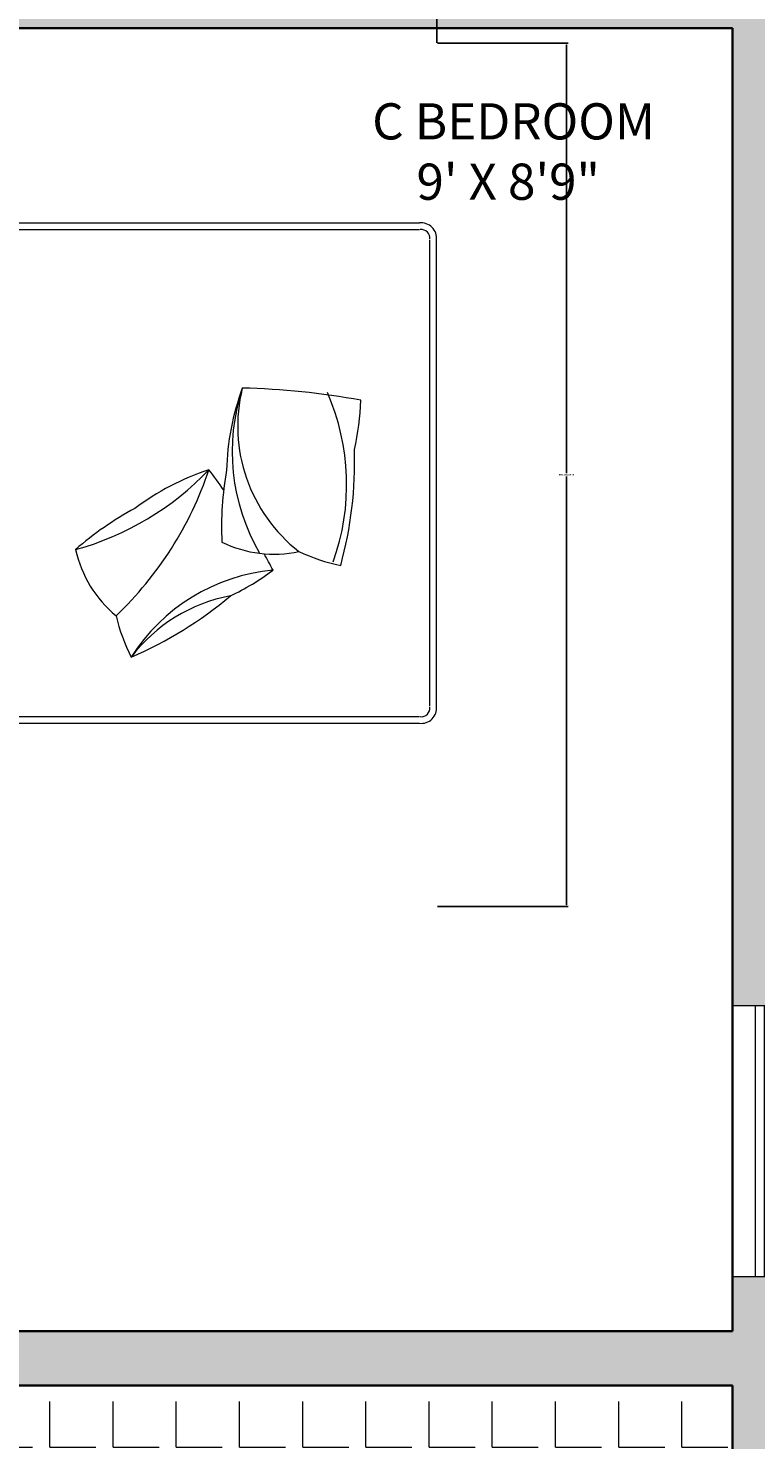
# Model space of a CAD drawing. Units: inches. Extents: x 2701 to 6846, y 811 to 2447.
# Tile 18 of 20: x 3008 to 3089, y 1300 to 1456. Entities that reach past the tile are written whole.
import ezdxf

# ---------------------------------------------------------------- set-up
doc = ezdxf.new("R2010")
doc.units = ezdxf.units.IN
for name, color, linetype, lineweight in [('A-ANNO-DIMS', 2, 'Continuous', 18), ('A-AREA-IDEN', 7, 'Continuous', 18), ('A-FLOR-PATT', 252, 'Continuous', 13), ('A-FURN', 8, 'Continuous', 13), ('A-GLAZ', 4, 'Continuous', 18), ('A-WALL', 7, 'Continuous', 35)]:
    doc.layers.add(name, color=color, linetype=linetype, lineweight=lineweight)
doc.layers.add('A-WALL-PATT', color=18, linetype='Continuous', lineweight=13, true_color=0x000000)
doc.styles.get("Standard").update_dxf_attribs({"font": 'arial.ttf'})
doc.dimstyles.get("Standard").update_dxf_attribs({"dimtxt": 0.18, "dimasz": 0.18, "dimexe": 0.18, "dimexo": 0.0625, "dimgap": 0.09, "dimtad": 0, "dimtih": 1, "dimtoh": 1, "dimdec": 4, "dimzin": 0, "dimdsep": 46, "dimtxsty": 'Standard', "dimcen": 0.09, "dimadec": 0, "dimazin": 0, "dimtfac": 1, "dimtdec": 4, "dimtofl": 0, "dimtmove": 0, "dimatfit": 3, "dimfxl": 1, "dimtolj": 1, "dimtzin": 0, "dimarcsym": 0})

# ---------------------------------------------------------------- blocks, each defined once
blk = doc.blocks.new('W1')
for p, q in [((3091.97, 1348.05), (3091.97, 1360.05)), ((3091.97, 1360.05), (3091.97, 1358.83)), ((3091.97, 1360.05), (3101.22, 1360.05)), ((3101.22, 1306.05), (3101.22, 1360.05)), ((3085.97, 1318.05), (3085.97, 1348.05)), ((3085.97, 1348.05), (3091.97, 1348.05)), ((3088.47, 1348.05), (3088.47, 1318.05)), ((3089.47, 1348.05), (3089.47, 1318.05)), ((3091.97, 1348.05), (3091.97, 1348.05)), ((3091.97, 1348.05), (3091.97, 1318.05)), ((3091.97, 1318.05), (3085.97, 1318.05)), ((3091.97, 1318.05), (3091.97, 1306.05)), ((3091.97, 1306.05), (3091.97, 1306.05)), ((3091.97, 1306.05), (3101.22, 1306.05))]:
    blk.add_line(p, q)
blk.add_circle((3096.65, 1332.84), 3.33)
at = {"insert": (3097.78, 1330.51), "char_height": 2.5, "attachment_point": 7, "rotation": 90}
blk.add_mtext('W1', dxfattribs=at)
blk = doc.blocks.new('A$C356F0359')
for p, q in [((0.5489, 2), (2.0492, 2)), ((0.5489, 1.9489), (0.5489, 2)), ((2.0492, 1.9489), (2.0492, 2)), ((0.4398, 1.9801), (0.0598, 1.9801)), ((0.4398, 1.9601), (0.0598, 1.9601)), ((2.0492, 1.9489), (0.5489, 1.9489)), ((2.5283, 1.9801), (2.1483, 1.9801)), ((2.5283, 1.9601), (2.1483, 1.9601)), ((-0.0002, 1.9201), (-0.0002, 1.5401)), ((0.0198, 1.9201), (0.0198, 1.5401)), ((0.4798, 1.5401), (0.4798, 1.9201)), ((0.4998, 1.5401), (0.4998, 1.9201)), ((1.998, 1.9289), (0.6001, 1.9289)), ((2.0883, 1.9201), (2.0883, 1.5401)), ((2.1083, 1.9201), (2.1083, 1.5401)), ((2.5683, 1.5401), (2.5683, 1.9201)), ((2.5883, 1.5401), (2.5883, 1.9201)), ((0.1539, 1.5681), (0.1539, 1.8777)), ((0.2725, 1.8879), (0.2702, 1.8856)), ((0.2702, 1.8856), (0.2702, 1.7279)), ((0.2725, 1.8879), (0.4531, 1.8879)), ((0.3913, 1.8753), (0.277, 1.8753)), ((0.277, 1.8753), (0.277, 1.8147)), ((0.3913, 1.8147), (0.3913, 1.8753)), ((0.4016, 1.8787), (0.4062, 1.8845)), ((0.4016, 1.7404), (0.4016, 1.8787)), ((0.4062, 1.881), (0.405, 1.8765)), ((0.405, 1.8765), (0.4153, 1.8662)), ((0.405, 1.8765), (0.405, 1.8456)), ((0.4062, 1.8845), (0.4405, 1.8845)), ((0.4108, 1.8833), (0.4062, 1.881)), ((0.4108, 1.8833), (0.4382, 1.8833)), ((0.4165, 1.8685), (0.4108, 1.8833)), ((0.4153, 1.8662), (0.4165, 1.8685)), ((0.4153, 1.8147), (0.4153, 1.8662)), ((0.4325, 1.8685), (0.4165, 1.8685)), ((0.4325, 1.8685), (0.4382, 1.8833)), ((0.4336, 1.8662), (0.4325, 1.8685)), ((0.4439, 1.8765), (0.4336, 1.8662)), ((0.4336, 1.8147), (0.4336, 1.8662)), ((0.4382, 1.8833), (0.4428, 1.881)), ((0.4405, 1.8845), (0.4462, 1.8787)), ((0.4428, 1.881), (0.4439, 1.8765)), ((0.4439, 1.8765), (0.4439, 1.8456)), ((0.4462, 1.8787), (0.4462, 1.7416)), ((0.4531, 1.8879), (0.4553, 1.8856)), ((0.4553, 1.8856), (0.4553, 1.7279)), ((0.5489, 1.8977), (0.5489, 0.0512)), ((0.5689, 1.8977), (0.5689, 0.0512)), ((2.0292, 0.0512), (2.0292, 1.8977)), ((2.0492, 0.0512), (2.0492, 1.8977)), ((2.3306, 1.5822), (2.3306, 1.8917)), ((0.405, 1.8456), (0.4073, 1.8399)), ((0.4073, 1.8399), (0.4108, 1.8342)), ((0.4108, 1.8342), (0.4119, 1.8262)), ((0.4119, 1.8262), (0.4119, 1.8147)), ((0.4382, 1.8342), (0.4371, 1.8262)), ((0.4371, 1.8262), (0.4371, 1.8147)), ((0.4416, 1.8399), (0.4382, 1.8342)), ((0.4439, 1.8456), (0.4416, 1.8399)), ((0.277, 1.8147), (0.3913, 1.8147)), ((0.277, 1.7885), (0.277, 1.7679)), ((0.3445, 1.7885), (0.277, 1.7885)), ((0.3913, 1.8125), (0.2816, 1.8125)), ((0.2816, 1.8125), (0.2816, 1.801)), ((0.2816, 1.801), (0.3913, 1.801)), ((0.2885, 1.7862), (0.2885, 1.7827)), ((0.2919, 1.7862), (0.2885, 1.7862)), ((0.2885, 1.7827), (0.2919, 1.7827)), ((0.2907, 1.8125), (0.2907, 1.801)), ((0.2919, 1.7827), (0.2919, 1.7862)), ((0.2999, 1.8125), (0.2999, 1.801)), ((0.309, 1.8125), (0.309, 1.801)), ((0.3125, 1.7862), (0.309, 1.7862)), ((0.309, 1.7862), (0.309, 1.7827)), ((0.309, 1.7827), (0.3125, 1.7827)), ((0.3125, 1.7827), (0.3125, 1.7862)), ((0.3182, 1.8125), (0.3182, 1.801)), ((0.3273, 1.8125), (0.3273, 1.801)), ((0.333, 1.7862), (0.3296, 1.7862)), ((0.3296, 1.7862), (0.3296, 1.7827)), ((0.3296, 1.7827), (0.333, 1.7827)), ((0.333, 1.7827), (0.333, 1.7862)), ((0.3365, 1.8125), (0.3365, 1.801)), ((0.3445, 1.7679), (0.3445, 1.7885)), ((0.3548, 1.7759), (0.3548, 1.7827)), ((0.3548, 1.7827), (0.3639, 1.7827)), ((0.3639, 1.7827), (0.3639, 1.7759)), ((0.3685, 1.7827), (0.3776, 1.7827)), ((0.3685, 1.7759), (0.3685, 1.7827)), ((0.3776, 1.7827), (0.3776, 1.7759)), ((0.3822, 1.7759), (0.3822, 1.7827)), ((0.3822, 1.7827), (0.3913, 1.7827)), ((0.3913, 1.801), (0.3913, 1.8125)), ((0.3913, 1.7827), (0.3913, 1.7759)), ((0.405, 1.7736), (0.4073, 1.7793)), ((0.4073, 1.7793), (0.4108, 1.785)), ((0.4108, 1.785), (0.4119, 1.793)), ((0.4119, 1.793), (0.4119, 1.8147)), ((0.4153, 1.8147), (0.4153, 1.753)), ((0.4336, 1.8147), (0.4336, 1.753)), ((0.4371, 1.793), (0.4371, 1.8147)), ((0.4382, 1.785), (0.4371, 1.793)), ((0.4416, 1.7793), (0.4382, 1.785)), ((0.4439, 1.7736), (0.4416, 1.7793)), ((0.277, 1.7679), (0.3445, 1.7679)), ((0.2782, 1.7622), (0.2782, 1.7576)), ((0.2896, 1.7622), (0.2782, 1.7622)), ((0.2782, 1.7576), (0.2896, 1.7576)), ((0.2782, 1.745), (0.2896, 1.745)), ((0.2782, 1.7382), (0.2782, 1.745)), ((0.2896, 1.7382), (0.2782, 1.7382)), ((0.2919, 1.7736), (0.2885, 1.7736)), ((0.2885, 1.7736), (0.2885, 1.7702)), ((0.2885, 1.7702), (0.2919, 1.7702)), ((0.2896, 1.7576), (0.2896, 1.7622)), ((0.2896, 1.745), (0.2896, 1.7382)), ((0.2919, 1.7702), (0.2919, 1.7736)), ((0.2942, 1.7622), (0.2942, 1.7576)), ((0.3056, 1.7622), (0.2942, 1.7622)), ((0.2942, 1.7576), (0.3056, 1.7576)), ((0.2942, 1.745), (0.3056, 1.745)), ((0.2942, 1.7382), (0.2942, 1.745)), ((0.3056, 1.7382), (0.2942, 1.7382)), ((0.3056, 1.7576), (0.3056, 1.7622)), ((0.3056, 1.745), (0.3056, 1.7382)), ((0.3125, 1.7736), (0.309, 1.7736)), ((0.309, 1.7736), (0.309, 1.7702)), ((0.309, 1.7702), (0.3125, 1.7702)), ((0.3102, 1.7622), (0.3102, 1.7576)), ((0.3216, 1.7622), (0.3102, 1.7622)), ((0.3102, 1.7576), (0.3216, 1.7576)), ((0.3102, 1.745), (0.3216, 1.745)), ((0.3102, 1.7382), (0.3102, 1.745)), ((0.3216, 1.7382), (0.3102, 1.7382)), ((0.3125, 1.7702), (0.3125, 1.7736)), ((0.3216, 1.7576), (0.3216, 1.7622)), ((0.3216, 1.745), (0.3216, 1.7382)), ((0.3376, 1.7622), (0.3262, 1.7622)), ((0.3262, 1.7622), (0.3262, 1.7576)), ((0.3262, 1.7576), (0.3376, 1.7576)), ((0.3262, 1.7382), (0.3262, 1.745)), ((0.3262, 1.745), (0.3376, 1.745)), ((0.3376, 1.7382), (0.3262, 1.7382)), ((0.333, 1.7736), (0.3296, 1.7736)), ((0.3296, 1.7736), (0.3296, 1.7702)), ((0.3296, 1.7702), (0.333, 1.7702)), ((0.333, 1.7702), (0.333, 1.7736)), ((0.3376, 1.7576), (0.3376, 1.7622)), ((0.3376, 1.745), (0.3376, 1.7382)), ((0.3639, 1.7759), (0.3548, 1.7759)), ((0.3548, 1.7633), (0.3548, 1.7702)), ((0.3548, 1.7702), (0.3639, 1.7702)), ((0.3639, 1.7633), (0.3548, 1.7633)), ((0.3548, 1.7564), (0.3639, 1.7564)), ((0.3548, 1.7496), (0.3548, 1.7564)), ((0.3639, 1.7496), (0.3548, 1.7496)), ((0.3548, 1.737), (0.3548, 1.7439)), ((0.3548, 1.7439), (0.3639, 1.7439)), ((0.3639, 1.737), (0.3548, 1.737)), ((0.3639, 1.7702), (0.3639, 1.7633)), ((0.3639, 1.7564), (0.3639, 1.7496)), ((0.3639, 1.7439), (0.3639, 1.737)), ((0.3776, 1.7759), (0.3685, 1.7759)), ((0.3685, 1.7633), (0.3685, 1.7702)), ((0.3685, 1.7702), (0.3776, 1.7702)), ((0.3776, 1.7633), (0.3685, 1.7633)), ((0.3685, 1.7564), (0.3776, 1.7564)), ((0.3685, 1.7496), (0.3685, 1.7564)), ((0.3776, 1.7496), (0.3685, 1.7496)), ((0.3685, 1.737), (0.3685, 1.7439)), ((0.3685, 1.7439), (0.3776, 1.7439)), ((0.3776, 1.737), (0.3685, 1.737)), ((0.3776, 1.7702), (0.3776, 1.7633)), ((0.3776, 1.7564), (0.3776, 1.7496)), ((0.3776, 1.7439), (0.3776, 1.737)), ((0.3913, 1.7759), (0.3822, 1.7759)), ((0.3822, 1.7633), (0.3822, 1.7702)), ((0.3822, 1.7702), (0.3913, 1.7702)), ((0.3913, 1.7633), (0.3822, 1.7633)), ((0.3822, 1.7576), (0.3913, 1.7576)), ((0.3822, 1.7507), (0.3822, 1.7576)), ((0.3913, 1.7507), (0.3822, 1.7507)), ((0.3822, 1.7439), (0.3913, 1.7439)), ((0.3822, 1.737), (0.3822, 1.7439)), ((0.3913, 1.737), (0.3822, 1.737)), ((0.3913, 1.7702), (0.3913, 1.7633)), ((0.3913, 1.7576), (0.3913, 1.7507)), ((0.3913, 1.7439), (0.3913, 1.737)), ((0.4073, 1.7347), (0.4016, 1.7404)), ((0.405, 1.7427), (0.405, 1.7736)), ((0.405, 1.7427), (0.4153, 1.753)), ((0.4062, 1.7382), (0.405, 1.7427)), ((0.4108, 1.7359), (0.4062, 1.7382)), ((0.4165, 1.7507), (0.4108, 1.7359)), ((0.4108, 1.7359), (0.4234, 1.7359)), ((0.4153, 1.753), (0.4165, 1.7507)), ((0.4325, 1.7507), (0.4165, 1.7507)), ((0.4233, 1.7393), (0.4235, 1.7294)), ((0.4268, 1.7393), (0.4233, 1.7393)), ((0.4274, 1.7301), (0.4268, 1.7393)), ((0.427, 1.7359), (0.4382, 1.7359)), ((0.4336, 1.753), (0.4325, 1.7507)), ((0.4325, 1.7507), (0.4382, 1.7359)), ((0.4439, 1.7427), (0.4336, 1.753)), ((0.4382, 1.7359), (0.4428, 1.7382)), ((0.4462, 1.7416), (0.4405, 1.7347)), ((0.4428, 1.7382), (0.4439, 1.7427)), ((0.4439, 1.7427), (0.4439, 1.7736)), ((0.4622, 1.7459), (0.4553, 1.7484)), ((0.4553, 1.7439), (0.4604, 1.7425)), ((0.4604, 1.7425), (0.465, 1.7388)), ((0.4654, 1.7427), (0.4622, 1.7459)), ((0.465, 1.7388), (0.4662, 1.7372)), ((0.4678, 1.7405), (0.4654, 1.7427)), ((0.4662, 1.7372), (0.4686, 1.7374)), ((0.4686, 1.7374), (0.4662, 1.735)), ((0.4721, 1.7421), (0.4678, 1.7405)), ((0.4741, 1.7401), (0.4721, 1.7421)), ((0.4725, 1.7366), (0.4741, 1.7401)), ((0.4753, 1.7388), (0.4725, 1.7366)), ((0.4783, 1.7356), (0.4753, 1.7388)), ((2.4819, 1.7366), (2.1818, 1.7366)), ((0.3052, 1.7226), (0.0051, 1.7226)), ((0.2702, 1.7279), (0.2725, 1.7256)), ((0.4244, 1.7256), (0.2725, 1.7256)), ((0.4234, 1.7347), (0.4073, 1.7347)), ((0.4235, 1.7294), (0.4263, 1.7179)), ((0.4263, 1.7179), (0.429, 1.707)), ((0.427, 1.697), (0.4265, 1.6915)), ((0.4295, 1.6996), (0.427, 1.697)), ((0.4405, 1.7347), (0.4271, 1.7347)), ((0.429, 1.7227), (0.4274, 1.7301)), ((0.4531, 1.7256), (0.4284, 1.7256)), ((0.429, 1.707), (0.4288, 1.701)), ((0.4288, 1.701), (0.4295, 1.6996)), ((0.4318, 1.7119), (0.429, 1.7227)), ((0.4325, 1.7063), (0.4318, 1.7119)), ((0.4323, 1.7003), (0.4325, 1.7063)), ((0.4364, 1.6973), (0.4323, 1.7003)), ((0.4355, 1.6919), (0.4364, 1.6973)), ((0.4553, 1.7279), (0.4531, 1.7256)), ((0.4662, 1.735), (0.4755, 1.7268)), ((0.4755, 1.7268), (0.4906, 1.7139)), ((0.4759, 1.729), (0.4783, 1.7356)), ((0.4821, 1.7322), (0.4759, 1.729)), ((0.4874, 1.7272), (0.4821, 1.7322)), ((0.4862, 1.7199), (0.4874, 1.7272)), ((0.4914, 1.7231), (0.4862, 1.7199)), ((0.4908, 1.7135), (0.4984, 1.6917)), ((0.4958, 1.7185), (0.4914, 1.7231)), ((0.494, 1.7135), (0.4958, 1.7185)), ((0.501, 1.7142), (0.494, 1.7135)), ((0.4964, 1.7047), (0.5031, 1.7072)), ((0.5038, 1.7049), (0.4964, 1.7047)), ((0.5005, 1.695), (0.5054, 1.6996)), ((0.5068, 1.695), (0.5005, 1.695)), ((0.5031, 1.7072), (0.501, 1.7142)), ((0.5054, 1.6996), (0.5038, 1.7049)), ((0.5079, 1.6892), (0.5068, 1.695)), ((0.4265, 1.6915), (0.4332, 1.6903)), ((0.4332, 1.6903), (0.4267, 1.6864)), ((0.4267, 1.6864), (0.4272, 1.6801)), ((0.4272, 1.6801), (0.4346, 1.6794)), ((0.4346, 1.6794), (0.4281, 1.6744)), ((0.4281, 1.6744), (0.4311, 1.669)), ((0.4311, 1.669), (0.4381, 1.6704)), ((0.4381, 1.6704), (0.4348, 1.6639)), ((0.4348, 1.6639), (0.4383, 1.6598)), ((0.4367, 1.6774), (0.4355, 1.6919)), ((0.4455, 1.6663), (0.4367, 1.6774)), ((0.4383, 1.6598), (0.4436, 1.6637)), ((0.4436, 1.6637), (0.4427, 1.6575)), ((0.4427, 1.6575), (0.4471, 1.6547)), ((0.4577, 1.6598), (0.4455, 1.6663)), ((0.4471, 1.6547), (0.4526, 1.6593)), ((0.4526, 1.6593), (0.4519, 1.6517)), ((0.4519, 1.6517), (0.4568, 1.6503)), ((0.4568, 1.6503), (0.4598, 1.6565)), ((0.4716, 1.6586), (0.4577, 1.6598)), ((0.4598, 1.6565), (0.4626, 1.6503)), ((0.4665, 1.6498), (0.4681, 1.6565)), ((0.4681, 1.6565), (0.4707, 1.6491)), ((0.485, 1.6644), (0.4716, 1.6586)), ((0.4751, 1.6503), (0.4753, 1.6565)), ((0.4753, 1.6565), (0.4806, 1.6519)), ((0.4806, 1.6519), (0.4843, 1.6538)), ((0.4843, 1.6538), (0.4836, 1.6607)), ((0.4836, 1.6607), (0.4885, 1.6547)), ((0.4952, 1.6744), (0.485, 1.6644)), ((0.4885, 1.6547), (0.4922, 1.6579)), ((0.4922, 1.6579), (0.4894, 1.6642)), ((0.4894, 1.6642), (0.4959, 1.6614)), ((0.4984, 1.6917), (0.4952, 1.6744)), ((0.4957, 1.6704), (0.5024, 1.6683)), ((0.4989, 1.6642), (0.4957, 1.6704)), ((0.4959, 1.6614), (0.4989, 1.6642)), ((0.5042, 1.673), (0.4987, 1.6792)), ((0.4987, 1.6792), (0.5058, 1.679)), ((0.5008, 1.6871), (0.5079, 1.6892)), ((0.5068, 1.6836), (0.5008, 1.6871)), ((0.5024, 1.6683), (0.5042, 1.673)), ((0.5058, 1.679), (0.5068, 1.6836)), ((0.4626, 1.6503), (0.4665, 1.6498)), ((0.4707, 1.6491), (0.4751, 1.6503)), ((0.0598, 1.5001), (0.4398, 1.5001)), ((2.1483, 1.5001), (2.5283, 1.5001)), ((0.0598, 1.4801), (0.4398, 1.4801)), ((2.1483, 1.4801), (2.5283, 1.4801)), ((0.6001, 0.02), (1.998, 0.02)), ((0.6001, 0), (1.998, 0))]:
    blk.add_line(p, q)
at = {"linetype": 'ByBlock'}
for p, q in [((0.6001, 1.9147), (1.282, 1.9147)), ((0.6001, 1.6759), (0.6001, 1.9147)), ((1.282, 1.9147), (1.282, 1.6759)), ((1.3161, 1.9147), (1.998, 1.9147)), ((1.3161, 1.6759), (1.3161, 1.9147)), ((1.998, 1.9147), (1.998, 1.6759)), ((1.282, 1.6759), (0.6001, 1.6759)), ((1.998, 1.6759), (1.3161, 1.6759)), ((1.0687, 1.6418), (0.5489, 1.6418)), ((1.4185, 1.5053), (0.5489, 1.5053))]:
    blk.add_line(p, q, dxfattribs=at)
for centre in [(0.1539, 1.7226), (2.3306, 1.7366)]:
    blk.add_circle(centre, 0.12, dxfattribs=at)
for centre in [(0.1539, 1.7226), (2.3306, 1.7366)]:
    blk.add_circle(centre, 0.06)
for centre, radius, start, end in [((0.0598, 1.9201), 0.06, 90, 180), ((0.0598, 1.9201), 0.04, 90, 180), ((0.4398, 1.9201), 0.06, 0, 90), ((0.4398, 1.9201), 0.04, 0, 90), ((0.6001, 1.8977), 0.0512, 90, 180), ((1.998, 1.8977), 0.0512, 0, 90), ((2.1483, 1.9201), 0.06, 90, 180), ((2.1483, 1.9201), 0.04, 90, 180), ((2.5283, 1.9201), 0.06, 0, 90), ((2.5283, 1.9201), 0.04, 0, 90), ((0.6001, 1.8977), 0.0312, 90, 180), ((1.998, 1.8977), 0.0312, 0, 90), ((0.0598, 1.5401), 0.06, 180, 270), ((0.0598, 1.5401), 0.04, 180, 270), ((0.4398, 1.5401), 0.04, 270, 0), ((0.4398, 1.5401), 0.06, 270, 0), ((2.1483, 1.5401), 0.06, 180, 270), ((2.1483, 1.5401), 0.04, 180, 270), ((2.5283, 1.5401), 0.06, 270, 0), ((2.5283, 1.5401), 0.04, 270, 0), ((1.1471, 0.7332), 0.3575, 102.4782, 140.4625), ((1.9086, 1.3124), 0.8697, 195.336, 226.4193), ((0.3249, 0.4335), 0.9879, 28.4971, 41.0566), ((0.9965, 0.4273), 0.548, 103.2034, 117.0362), ((1.6529, 1.7059), 1.0798, 223.6306, 251.4288), ((0.4451, 0.4375), 0.5655, 5.3391, 57.6895), ((0.4517, 0.5274), 0.4879, 10.6986, 52.6864), ((1.8195, 1.3719), 1.1652, 203.0642, 220.3209), ((0.5617, 0.4344), 0.7874, 18.3527, 36.6851), ((-0.021, 2.4319), 2.1977, 305.2966, 307.2418), ((1.4135, 0.487), 0.3575, 154.0418, 192.0262), ((1.1372, -0.3434), 0.9879, 80.0607, 92.6202), ((1.5949, 0.9312), 0.734, 205.259, 216.9351), ((1.3641, 0.0041), 0.6085, 71.81, 120.1351), ((1.44, 0.1186), 0.4774, 76.1849, 142.0017), ((1.2836, -0.1573), 0.7874, 69.9163, 88.2487), ((-0.6432, 0.628), 2.1977, 349.4884, 358.8054), ((-0.021, 2.4319), 2.1977, 297.9248, 299.3793), ((1.5595, 0.1789), 0.548, 154.767, 168.5998), ((1.2647, 0.9578), 0.6885, 250.2936, 293.6414), ((1.3312, 1.4107), 1.1652, 254.6278, 271.8845), ((1.5368, 0.9609), 0.734, 256.8226, 268.4988), ((0.5943, 0.0454), 0.0458, 172.7599, 277.2401), ((0.5943, 0.0454), 0.0258, 172.7599, 277.2401), ((2.0038, 0.0454), 0.0458, 262.7599, 7.2401), ((2.0038, 0.0454), 0.0258, 262.7599, 7.2401)]:
    blk.add_arc(centre, radius, start, end)
for centre, radius, start, end in [((0.1906, 1.7953), 0.4265, 343.7398, 16.2602), ((1.6914, 1.7953), 0.4265, 163.7398, 196.2602), ((0.9067, 1.7953), 0.4265, 343.7398, 16.2602), ((2.4075, 1.7953), 0.4265, 163.7398, 196.2602), ((0.9303, 0.657), 0.9853, 61.4328, 88.1261), ((1.0826, 0.5712), 1.0706, 72.1966, 90.7418), ((2.1368, 4.5996), 3.0955, 256.4201, 268.3789), ((2.0056, 2.7745), 1.3903, 244.2427, 271.7984)]:
    blk.add_arc(centre, radius, start, end, dxfattribs=at)
blk = doc.blocks.new('*D34')
at = {"layer": 'A-ANNO-DIMS', "color": 0, "lineweight": -2, "transparency": 16777216}
for p, q in [((3085.97, 1305.99), (3085.97, 1297.77)), ((3101.22, 1305.99), (3101.22, 1297.77)), ((3086.15, 1297.95), (3093.38, 1297.95)), ((3101.04, 1297.95), (3093.81, 1297.95))]:
    blk.add_line(p, q, dxfattribs=at)
at = {"layer": 'A-ANNO-DIMS', "color": 0, "transparency": 16777216}
for points in [[(3086.15, 1297.98), (3086.15, 1297.92), (3085.97, 1297.95)], [(3101.04, 1297.98), (3101.04, 1297.92), (3101.22, 1297.95)]]:
    blk.add_solid(points, dxfattribs=at)
at = {"layer": 'Defpoints', "color": 0, "transparency": 16777216}
for p in [(3085.97, 1306.05), (3101.22, 1306.05), (3101.22, 1297.95)]:
    blk.add_point(p, dxfattribs=at)
at = {"layer": 'A-ANNO-DIMS', "color": 0, "transparency": 16777216, "insert": (3093.59, 1297.95), "char_height": 0.18, "attachment_point": 5}
blk.add_mtext('\\A1;15', dxfattribs=at)
blk = doc.blocks.new('*D51')
at = {"layer": 'A-ANNO-DIMS', "color": 0, "lineweight": -2, "transparency": 16777216}
for p, q in [((3053.38, 1454.39), (3067.81, 1454.39)), ((3067.63, 1454.21), (3067.63, 1406.88)), ((3067.63, 1359.18), (3067.63, 1406.51)), ((3053.38, 1359), (3067.81, 1359))]:
    blk.add_line(p, q, dxfattribs=at)
at = {"layer": 'A-ANNO-DIMS', "color": 0, "transparency": 16777216}
for points in [[(3067.6, 1454.21), (3067.66, 1454.21), (3067.63, 1454.39)], [(3067.6, 1359.18), (3067.66, 1359.18), (3067.63, 1359)]]:
    blk.add_solid(points, dxfattribs=at)
at = {"layer": 'Defpoints', "color": 0, "transparency": 16777216}
for p in [(3053.32, 1454.39), (3067.63, 1454.39), (3053.32, 1359)]:
    blk.add_point(p, dxfattribs=at)
at = {"layer": 'A-ANNO-DIMS', "color": 0, "transparency": 16777216, "insert": (3067.63, 1406.69), "char_height": 0.18, "attachment_point": 5}
blk.add_mtext('\\A1;BED GROUP 95', dxfattribs=at)
blk = doc.blocks.new('*D52')
at = {"layer": 'A-ANNO-DIMS', "color": 0, "lineweight": -2, "transparency": 16777216}
for p, q in [((2979.55, 1454.45), (2979.55, 1468.88)), ((2979.73, 1468.7), (3016.22, 1468.7)), ((3053.14, 1468.7), (3016.65, 1468.7)), ((3053.32, 1454.45), (3053.32, 1468.88))]:
    blk.add_line(p, q, dxfattribs=at)
at = {"layer": 'A-ANNO-DIMS', "color": 0, "transparency": 16777216}
for points in [[(2979.73, 1468.73), (2979.73, 1468.67), (2979.55, 1468.7)], [(3053.14, 1468.73), (3053.14, 1468.67), (3053.32, 1468.7)]]:
    blk.add_solid(points, dxfattribs=at)
at = {"layer": 'Defpoints', "color": 0, "transparency": 16777216}
for p in [(2979.55, 1468.7), (2979.55, 1454.39), (3053.32, 1454.39)]:
    blk.add_point(p, dxfattribs=at)
at = {"layer": 'A-ANNO-DIMS', "color": 0, "transparency": 16777216, "insert": (3016.44, 1468.7), "char_height": 0.18, "attachment_point": 5}
blk.add_mtext('\\A1;74', dxfattribs=at)

msp = doc.modelspace()

# ---------------------------------------------------------------- hatches: boundary and pattern name
at = {"layer": 'A-FLOR-PATT'}
h = msp.add_hatch(dxfattribs=at)
h.set_pattern_fill('ANGLE', color=256)
h.set_pattern_definition([(0, (0, 0), (0, 6.985), [5.08, -1.905]), (90, (0, 0), (-6.985, 4e-16), [5.08, -1.905])])
h.paths.add_polyline_path([(2841.81, 1296.51, -0.109453), (2842.61, 1300.13, -0.102375), (2844.98, 1303.3, -0.093743), (2848.43, 1305.37, -0.062463), (2851.37, 1306.05), (2785.97, 1306.05), (2785.97, 1258.05), (2827.97, 1258.05), (2827.97, 1256.41), (2829.45, 1256.41, -0.394827), (2854.75, 1283.45), (2856.49, 1283.45), (2856.49, 1256.41), (2857.97, 1256.41), (2857.97, 1258.05), (2863.97, 1258.05), (2863.97, 1306.05), (2853.87, 1306.05, -0.062463), (2856.81, 1305.37, -0.093743), (2860.26, 1303.3, -0.102375), (2862.62, 1300.13, -0.109453), (2863.42, 1296.51, -0.109453), (2862.62, 1292.89, -0.102375), (2860.26, 1289.72, -0.093738), (2856.81, 1287.65, -0.088425), (2852.62, 1286.91, -0.088425), (2848.43, 1287.65, -0.093738), (2844.98, 1289.72, -0.102375), (2842.61, 1292.89, -0.109453)])
h.paths.add_polyline_path([(2805.21, 1273.88, -0.141745), (2808.32, 1271.77, -0.184983), (2809.77, 1267.97, -0.184983), (2808.32, 1264.18, -0.141745), (2805.21, 1262.07, -0.152244), (2799.99, 1261.8, -0.025614), (2799.37, 1261.95), (2794.37, 1263.42), (2794.36, 1263.41, -0.111242), (2793.99, 1261.92, -0.033889), (2793.11, 1260.11, -0.286745), (2792.38, 1259.65), (2787.58, 1259.65, -0.414214), (2787.15, 1260.08), (2787.15, 1267.97), (2787.15, 1275.87, -0.414214), (2787.58, 1276.3), (2792.38, 1276.3, -0.286745), (2793.11, 1275.83, -0.033889), (2793.99, 1274.03, -0.105104), (2794.36, 1272.63), (2794.37, 1272.53), (2799.37, 1274, -0.025614), (2799.99, 1274.15, -0.152244)], flags=16)
h.paths.add_polyline_path([(2804.68, 1272.34, -0.144945), (2807.09, 1270.71, -0.0358), (2807.45, 1270.25, -0.133285), (2807.89, 1268.61), (2807.89, 1267.97), (2807.89, 1267.34, -0.133285), (2807.45, 1265.7, -0.0358), (2807.09, 1265.24, -0.144945), (2804.68, 1263.61, -0.155404), (2800.34, 1263.39, -0.364511), (2796.49, 1267.97, -0.364511), (2800.34, 1272.56, -0.155404)], flags=0)
h.paths.add_polyline_path([(2800.02, 1268.9, 0.169298), (2799.13, 1268.12, 0.076667), (2799.1, 1267.97, 0.076667), (2799.13, 1267.83, 0.169298), (2800.02, 1267.05, 0.305219), (2800.37, 1267.16, 0.169535), (2800.65, 1267.97, 0.169535), (2800.37, 1268.79, 0.305219)], flags=0)
h.paths.add_polyline_path([(2971.97, 1456.05), (2923.97, 1456.05), (2923.97, 1408.05), (2922.33, 1408.05), (2922.33, 1406.57, -0.394827), (2949.37, 1381.27), (2949.37, 1379.53), (2922.33, 1379.53), (2922.33, 1378.05), (2923.97, 1378.05), (2923.97, 1372.05), (2971.97, 1372.05)])
h.paths.add_polyline_path([(2939.82, 1436.53, -0.141745), (2937.71, 1433.42, -0.184983), (2933.91, 1431.97, -0.184983), (2930.12, 1433.42, -0.141745), (2928.01, 1436.53, -0.152244), (2927.74, 1441.75, -0.025614), (2927.89, 1442.37), (2929.36, 1447.38), (2929.35, 1447.38, -0.111242), (2927.86, 1447.75, -0.033889), (2926.05, 1448.63, -0.286745), (2925.59, 1449.37), (2925.59, 1454.16, -0.414214), (2926.02, 1454.59), (2933.91, 1454.59), (2941.81, 1454.59, -0.414207), (2942.24, 1454.16), (2942.24, 1449.37, -0.286745), (2941.78, 1448.63, -0.033889), (2939.97, 1447.75, -0.105104), (2938.57, 1447.38), (2938.47, 1447.38), (2939.94, 1442.37, -0.025614), (2940.09, 1441.75, -0.152244)], flags=16)
h.paths.add_polyline_path([(2938.28, 1437.06, -0.144945), (2936.65, 1434.65, -0.0358), (2936.19, 1434.29, -0.133285), (2934.55, 1433.85), (2933.91, 1433.85), (2933.28, 1433.85, -0.133285), (2931.64, 1434.29, -0.0358), (2931.18, 1434.65, -0.144945), (2929.55, 1437.06, -0.155404), (2929.33, 1441.4, -0.364511), (2933.91, 1445.26, -0.364511), (2938.5, 1441.4, -0.155404)], flags=0)
h.paths.add_polyline_path([(2969.16, 1392.04, -0.093743), (2971.22, 1388.6, -0.088421), (2971.97, 1384.4, -0.088421), (2971.22, 1380.21, -0.093743), (2969.16, 1376.76, -0.102375), (2965.99, 1374.4, -0.109453), (2962.37, 1373.6, -0.109453), (2958.75, 1374.4, -0.102375), (2955.58, 1376.76, -0.093738), (2953.51, 1380.21, -0.088425), (2952.76, 1384.4, -0.088425), (2953.51, 1388.6, -0.093738), (2955.58, 1392.04, -0.102375), (2958.75, 1394.41, -0.109453), (2962.37, 1395.21, -0.109453), (2965.99, 1394.41, -0.102375)], flags=0)
edge = h.paths.add_edge_path(flags=16)
edge.add_arc((2961.07, 1384.86), 10.2, 20.2132, 41.6336, ccw=False)
edge.add_spline(control_points=[(2970.65, 1388.38), (2970.46, 1387.83), (2970, 1386.48), (2971.44, 1384.4), (2969.87, 1382.34), (2970.41, 1381.01), (2970.65, 1380.43)], knot_values=[0, 0, 0, 0, 0.041109, 0.100337, 0.155913, 0.199586, 0.199586, 0.199586, 0.199586], degree=3, periodic=0)
edge.add_arc((2961.07, 1383.95), 10.2, 318.3664, 339.7868, ccw=False)
edge.add_arc((2961.86, 1383.25), 9.15, 294.9853, 318.3664, ccw=False)
edge.add_arc((2962.37, 1382.17), 7.95, 270, 294.9853, ccw=False)
edge.add_arc((2962.37, 1382.17), 7.95, 245.0147, 270, ccw=False)
edge.add_arc((2962.87, 1383.25), 9.15, 221.6336, 245.0147, ccw=False)
edge.add_arc((2963.66, 1383.95), 10.2, 200.213, 221.6336, ccw=False)
edge.add_arc((2964.89, 1384.4), 11.51, 180, 200.213, ccw=False)
edge.add_arc((2964.89, 1384.4), 11.51, 159.787, 180, ccw=False)
edge.add_arc((2963.66, 1384.86), 10.2, 138.3664, 159.787, ccw=False)
edge.add_arc((2962.87, 1385.56), 9.15, 114.9853, 138.3664, ccw=False)
edge.add_arc((2962.37, 1386.64), 7.95, 90, 114.9853, ccw=False)
edge.add_arc((2962.37, 1386.64), 7.95, 65.0147, 90, ccw=False)
edge.add_arc((2961.86, 1385.56), 9.15, 41.6336, 65.0147, ccw=False)
h.paths.add_polyline_path([(2963.81, 1393.33, -0.126458), (2966.61, 1390.68, -0.141697), (2967.17, 1388.76), (2967.17, 1387.41, -1), (2969.57, 1387.41, -0.414214), (2968.37, 1386.21), (2963.57, 1385, 0.146218), (2963.31, 1384.66), (2968.97, 1385.64), (2968.97, 1383.15), (2963.32, 1384.13, 0.140312), (2963.57, 1383.8), (2968.37, 1382.6, -0.414214), (2969.57, 1381.4, -1), (2967.17, 1381.4), (2967.17, 1380.04, -0.149025), (2966.56, 1378.03, -0.012759), (2966.26, 1377.62, -0.106303), (2963.81, 1375.48, -0.126822), (2961.17, 1374.8, -0.126822), (2958.52, 1375.48, -0.106303), (2956.07, 1377.62, -0.085722), (2954.54, 1380.62, -0.075351), (2953.96, 1384.4, -0.075351), (2954.54, 1388.19, -0.085722), (2956.07, 1391.19, -0.106303), (2958.52, 1393.33, -0.126822), (2961.17, 1394.01, -0.126822)], flags=0)
h.paths.add_polyline_path([(2934.84, 1441.73, 0.169298), (2934.06, 1442.61, 0.076667), (2933.91, 1442.64, 0.076667), (2933.77, 1442.61, 0.169298), (2932.99, 1441.73, 0.305219), (2933.1, 1441.38, 0.169535), (2933.91, 1441.09, 0.169535), (2934.73, 1441.38, 0.305219)], flags=0)
h.paths.add_polyline_path([(2969.32, 1387.41, -1), (2967.42, 1387.41, -1)], flags=0)
h.paths.add_polyline_path([(2968.83, 1387.41, -1), (2967.91, 1387.41, -1)], flags=0)
h.paths.add_polyline_path([(2962.13, 1384.36, -1), (2960.21, 1384.36, -1)], flags=0)
h.paths.add_polyline_path([(2961.8, 1384.36, -1), (2960.54, 1384.36, -1)], flags=0)
h.paths.add_polyline_path([(2969.32, 1381.4, -1), (2967.42, 1381.4, -1)], flags=0)
h.paths.add_polyline_path([(2968.83, 1381.4, -1), (2967.91, 1381.4, -1)], flags=0)
h.paths.add_polyline_path([(3085.97, 1306.05), (3001.97, 1306.05), (3001.97, 1300.05), (3000.33, 1300.05), (3000.33, 1298.57), (3027.37, 1298.57), (3027.37, 1296.83, -0.394827), (3000.33, 1271.53), (3000.33, 1270.05), (3001.97, 1270.05), (3001.97, 1258.05), (3085.97, 1258.05)])
h.paths.add_polyline_path([(3033.33, 1274.44, -0.102375), (3035.7, 1271.27, -0.109453), (3036.5, 1267.65, -0.109453), (3035.7, 1264.04, -0.102375), (3033.33, 1260.86, -0.093743), (3029.88, 1258.8, -0.088421), (3025.69, 1258.05, -0.088421), (3021.5, 1258.8, -0.093743), (3018.05, 1260.86, -0.102375), (3015.69, 1264.04, -0.109453), (3014.89, 1267.65, -0.109453), (3015.69, 1271.27, -0.102375), (3018.05, 1274.44, -0.093738), (3021.5, 1276.51, -0.088425), (3025.69, 1277.26, -0.088425), (3029.88, 1276.51, -0.093738)], flags=0)
edge = h.paths.add_edge_path(flags=16)
edge.add_arc((3026.85, 1267.15), 9.15, 24.9853, 48.3664, ccw=False)
edge.add_arc((3027.93, 1267.65), 7.95, 0, 24.9853, ccw=False)
edge.add_arc((3027.93, 1267.65), 7.95, -24.9853, 0, ccw=False)
edge.add_arc((3026.85, 1268.16), 9.15, 311.6336, 335.0147, ccw=False)
edge.add_arc((3026.15, 1268.95), 10.2, 290.2132, 311.6336, ccw=False)
edge.add_spline(control_points=[(3029.67, 1259.38), (3029.09, 1259.61), (3027.76, 1260.15), (3025.7, 1258.59), (3023.62, 1260.02), (3022.27, 1259.56), (3021.71, 1259.38)], knot_values=[0, 0, 0, 0, 0.043673, 0.099248, 0.158477, 0.199586, 0.199586, 0.199586, 0.199586], degree=3, periodic=0)
edge.add_arc((3025.24, 1268.95), 10.2, 228.3664, 249.7868, ccw=False)
edge.add_arc((3024.54, 1268.16), 9.15, 204.9853, 228.3664, ccw=False)
edge.add_arc((3023.45, 1267.65), 7.95, 180, 204.9853, ccw=False)
edge.add_arc((3023.45, 1267.65), 7.95, 155.0147, 180, ccw=False)
edge.add_arc((3024.54, 1267.15), 9.15, 131.6336, 155.0147, ccw=False)
edge.add_arc((3025.24, 1266.36), 10.2, 110.213, 131.6336, ccw=False)
edge.add_arc((3025.69, 1265.13), 11.51, 90, 110.213, ccw=False)
edge.add_arc((3025.69, 1265.13), 11.51, 69.787, 90, ccw=False)
edge.add_arc((3026.15, 1266.36), 10.2, 48.3664, 69.787, ccw=False)
h.paths.add_polyline_path([(3032.48, 1273.95, -0.106303), (3034.62, 1271.5, -0.126822), (3035.3, 1268.85, -0.126822), (3034.62, 1266.21, -0.106303), (3032.48, 1263.76, -0.012759), (3032.07, 1263.46, -0.149025), (3030.06, 1262.85), (3028.69, 1262.85, -0.414214), (3029.89, 1261.65, -1), (3027.49, 1261.65), (3026.29, 1266.45, 0.140312), (3025.97, 1266.7), (3026.94, 1261.05), (3024.46, 1261.05), (3025.43, 1266.71, 0.146218), (3025.09, 1266.45), (3023.89, 1261.65, -1), (3021.49, 1261.65, -0.414214), (3022.69, 1262.85), (3021.34, 1262.85, -0.141697), (3019.41, 1263.41, -0.126458), (3016.77, 1266.21, -0.126822), (3016.09, 1268.85, -0.126822), (3016.77, 1271.5, -0.106303), (3018.91, 1273.95, -0.085722), (3021.91, 1275.48, -0.075351), (3025.69, 1276.06, -0.075351), (3029.47, 1275.48, -0.085722)], flags=0)
h.paths.add_polyline_path([(3072.36, 1280, -0.184983), (3076.16, 1281.46, -0.184983), (3079.96, 1280, -0.141745), (3082.07, 1276.9, -0.152244), (3082.34, 1271.68, -0.025614), (3082.19, 1271.05), (3080.72, 1266.05), (3080.82, 1266.04, -0.105104), (3082.22, 1265.68, -0.033889), (3084.02, 1264.8, -0.286745), (3084.49, 1264.06), (3084.49, 1259.26, -0.41422), (3084.06, 1258.84), (3076.16, 1258.84), (3068.27, 1258.84, -0.414214), (3067.84, 1259.26), (3067.84, 1264.06, -0.286745), (3068.3, 1264.8, -0.033889), (3070.1, 1265.68, -0.105104), (3071.51, 1266.04), (3071.61, 1266.05), (3070.13, 1271.05, -0.025614), (3069.98, 1271.68, -0.152244), (3070.26, 1276.9, -0.141745)], flags=16)
h.paths.add_polyline_path([(3073.43, 1278.77, -0.0358), (3073.88, 1279.13, -0.133285), (3075.53, 1279.58), (3076.16, 1279.58), (3076.8, 1279.58, -0.133285), (3078.44, 1279.13, -0.0358), (3078.9, 1278.77, -0.144945), (3080.53, 1276.36, -0.155404), (3080.75, 1272.03, -0.364511), (3076.16, 1268.17, -0.364511), (3071.57, 1272.03, -0.155404), (3071.8, 1276.36, -0.144945)], flags=0)
h.paths.add_polyline_path([(3026.7, 1268.85, -1), (3024.78, 1268.85, -1)], flags=0)
h.paths.add_polyline_path([(3026.37, 1268.85, -1), (3025.11, 1268.85, -1)], flags=0)
h.paths.add_polyline_path([(3075.27, 1271.62, 0.157677), (3076.02, 1270.81, 0.076667), (3076.16, 1270.78, 0.076667), (3076.3, 1270.81, 0.157677), (3077.06, 1271.62, 0.374626), (3076.98, 1272.05, 0.169535), (3076.16, 1272.33, 0.169535), (3075.35, 1272.05, 0.374626)], flags=0)
h.paths.add_polyline_path([(3029.65, 1261.65, -1), (3027.74, 1261.65, -1)], flags=0)
h.paths.add_polyline_path([(3029.15, 1261.65, -1), (3028.23, 1261.65, -1)], flags=0)
h.paths.add_polyline_path([(3023.65, 1261.65, -1), (3021.74, 1261.65, -1)], flags=0)
h.paths.add_polyline_path([(3023.15, 1261.65, -1), (3022.23, 1261.65, -1)], flags=0)
h.paths.add_polyline_path([(2810.57, 1281.22), (2833.31, 1281.22), (2833.31, 1296.43), (2810.57, 1296.43)], flags=24)
h.paths.add_polyline_path([(2937.55, 1410.24), (2960.21, 1410.24), (2960.21, 1425.45), (2937.55, 1425.45)], flags=24)
h.paths.add_polyline_path([(3043.23, 1273.1), (3065.89, 1273.1), (3065.89, 1288.31), (3043.23, 1288.31)], flags=24)
at = {"layer": 'A-WALL-PATT'}
h = msp.add_hatch(color=256, dxfattribs=at)
h.dxf.hatch_style = 1
h.paths.add_polyline_path([(3085.97, 1456.05), (3085.97, 1348.05), (3091.97, 1348.05), (3091.97, 1360.05), (3091.97, 1462.05), (2960.09, 1462.05), (2960.09, 1456.05), (2971.97, 1456.05), (2971.97, 1372.05), (2923.97, 1372.05), (2923.97, 1378.05), (2917.97, 1378.05), (2917.97, 1351.05), (2923.97, 1351.05), (2923.97, 1366.05), (2971.97, 1366.05), (2971.97, 1351.05), (2976.77, 1351.05), (2977.97, 1351.05), (2977.97, 1456.05)])
h.paths.add_polyline_path([(2779.97, 1462.05), (2779.97, 1342.05), (2785.97, 1342.05), (2785.97, 1456.05), (2917.97, 1456.05), (2917.97, 1408.05), (2922.33, 1408.05), (2923.97, 1408.05), (2923.97, 1456.05), (2937.09, 1456.05), (2937.09, 1462.05)])
h.paths.add_polyline_path([(2779.97, 1306.05), (2779.97, 1294.24), (2785.97, 1294.24), (2785.97, 1306.05), (2851.37, 1306.05, -0.025815), (2852.62, 1306.11, -0.025815), (2853.87, 1306.05), (2863.97, 1306.05), (2863.97, 1258.05), (2857.97, 1258.05), (2857.97, 1252.05), (2878.97, 1252.05), (2878.97, 1258.05), (2869.97, 1258.05), (2869.97, 1306.05), (2923.97, 1306.05), (2923.97, 1318.05), (2919.17, 1318.05), (2917.97, 1318.05), (2917.97, 1312.05), (2785.97, 1312.05), (2785.97, 1318.05), (2779.97, 1318.05)])
h.paths.add_polyline_path([(2785.97, 1252.05), (2827.97, 1252.05), (2827.97, 1256.41), (2827.97, 1258.05), (2785.97, 1258.05), (2785.97, 1271.24), (2779.97, 1271.24), (2779.97, 1174.05), (2785.97, 1174.05)])
h.paths.add_polyline_path([(2779.97, 1030.05), (2869.97, 1030.05), (2869.97, 1036.05), (2785.97, 1036.05), (2785.97, 1126.05), (2917.97, 1126.05), (2917.97, 1120.05), (2923.97, 1120.05), (2923.97, 1258.05), (2911.97, 1258.05), (2911.97, 1253.25), (2911.97, 1252.05), (2917.97, 1252.05), (2917.97, 1132.05), (2785.97, 1132.05), (2785.97, 1144.05), (2779.97, 1144.05)])
h.paths.add_polyline_path([(2935.97, 1030.05), (2935.97, 1033.05), (2935.97, 1036.05), (2923.97, 1036.05), (2923.97, 1087.05), (2919.17, 1087.05), (2917.97, 1087.05), (2917.97, 1036.05), (2893.97, 1036.05), (2893.97, 1030.05)])
h.paths.add_polyline_path([(2971.97, 1036.05), (2971.97, 1030.05), (3091.97, 1030.05), (3091.97, 1060.05), (3085.97, 1060.05), (3085.97, 1036.05)])
h.paths.add_polyline_path([(3085.97, 1084.05), (3091.97, 1084.05), (3091.97, 1096.05), (3091.97, 1268.89), (3085.97, 1268.89), (3085.97, 1258.05), (3001.97, 1258.05), (3001.97, 1270.05), (2995.97, 1270.05), (2995.97, 1252.05), (3085.97, 1252.05)])
h.paths.add_polyline_path([(3085.97, 1306.05), (3085.97, 1291.89), (3091.97, 1291.89), (3091.97, 1318.05), (3085.97, 1318.05), (3085.97, 1312.05), (2977.97, 1312.05), (2977.97, 1318.05), (2971.97, 1318.05), (2971.97, 1306.05), (2995.97, 1306.05), (2995.97, 1300.05), (3000.33, 1300.05), (3001.97, 1300.05), (3001.97, 1306.05)])

# ---------------------------------------------------------------- linework, layer by layer
at = {"layer": 'A-WALL'}
for p, q in [((3085.97, 1456.05), (2977.97, 1456.05)), ((3085.97, 1456.05), (3085.97, 1312.05)), ((3085.97, 1312.05), (2977.97, 1312.05)), ((3085.97, 1306.05), (3001.97, 1306.05)), ((3085.97, 1306.05), (3085.97, 1258.05))]:
    msp.add_line(p, q, dxfattribs=at)

# ---------------------------------------------------------------- block references
at = {"layer": 'A-FURN', "xscale": 36.85134703248138, "yscale": 36.85134703248138, "zscale": 36.85134703248138, "rotation": 90}
msp.add_blockref('A$C356F0359', (3053.26, 1359.01), dxfattribs=at)
at = {"layer": 'A-GLAZ'}
msp.add_blockref('W1', (0, 0), dxfattribs=at)

# ---------------------------------------------------------------- texts
at = {"layer": 'A-AREA-IDEN', "insert": (3046.16, 1447.76), "char_height": 4, "attachment_point": 1}
msp.add_mtext_dynamic_manual_height_columns('{\\fTimes New Roman|b0|i0|c0|p18;C BEDROOM\\P    9\' X 8\'9"}', width=57.2109, gutter_width=12.5, heights=[0], dxfattribs=at)

# ---------------------------------------------------------------- dimensions: what is measured, and where the dimension line sits
at = {"layer": 'A-ANNO-DIMS'}
dim = msp.add_linear_dim(base=(2979.55, 1468.7), p1=(3053.32, 1454.39), p2=(2979.55, 1454.39), angle=180, dimstyle='Standard', override={"dimdec": 0, "dimlfac": 1, "dimrnd": 0, "dimzin": 0, "dimdsep": 46, "dimlunit": 2}, dxfattribs=at)
dim.commit()
dim.dimension.update_dxf_attribs({"geometry": '*D52', "text_midpoint": (3016.44, 1468.7)})
dim = msp.add_linear_dim(base=(3067.63, 1454.39), p1=(3053.32, 1359), p2=(3053.32, 1454.39), angle=90, text='BED GROUP <>', dimstyle='Standard', override={"dimdec": 0, "dimlfac": 1, "dimrnd": 0, "dimzin": 0, "dimdsep": 46, "dimlunit": 2}, dxfattribs=at)
dim.commit()
dim.dimension.update_dxf_attribs({"geometry": '*D51', "text_midpoint": (3067.63, 1406.69)})
dim = msp.add_linear_dim(base=(3101.22, 1297.95), p1=(3085.97, 1306.05), p2=(3101.22, 1306.05), dimstyle='Standard', override={"dimdec": 0, "dimlfac": 1, "dimrnd": 0, "dimzin": 0, "dimdsep": 46, "dimlunit": 2}, dxfattribs=at)
dim.commit()
dim.dimension.update_dxf_attribs({"geometry": '*D34', "text_midpoint": (3093.59, 1297.95)})

doc.saveas('drawing.dxf')
